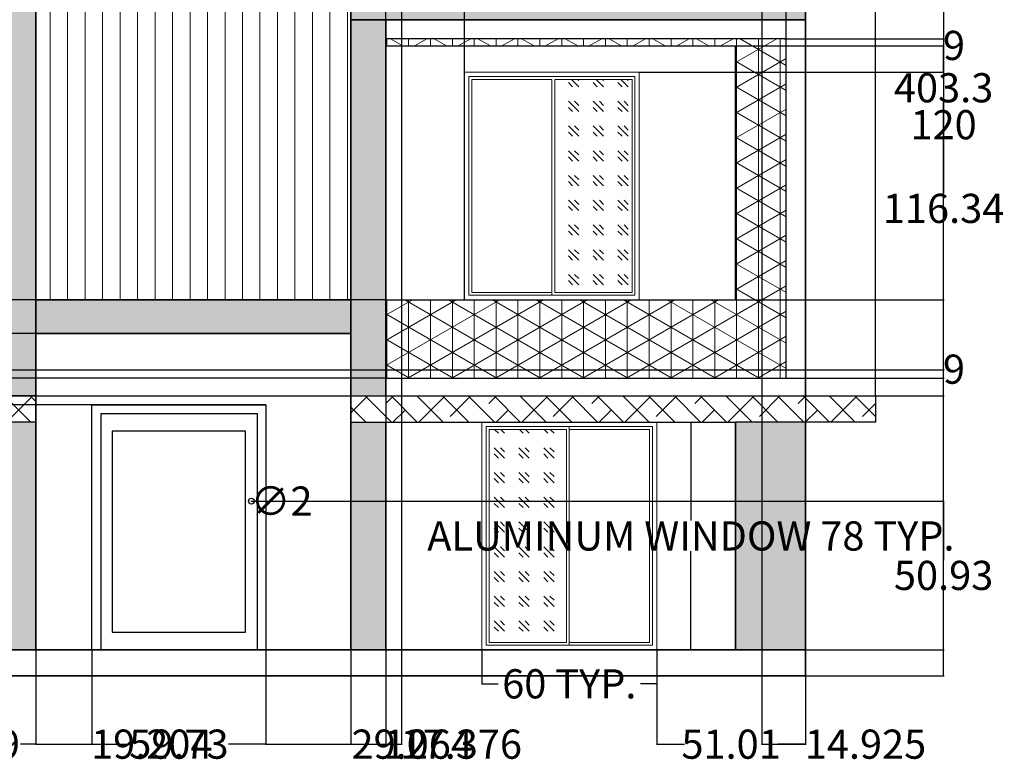
# Model space of a CAD drawing. Units: inches. Extents: x -37 to 519, y -28 to 435.
# Tile 2 of 3: x 182 to 519, y -28 to 227. Entities that reach past the tile are written whole.
import ezdxf

# ---------------------------------------------------------------- set-up
doc = ezdxf.new("R2010")
doc.units = ezdxf.units.IN
doc.header["$MEASUREMENT"] = 0
for name, color, linetype, lineweight in [('A-ANNO-DIMS', 2, 'Continuous', 18), ('A-DOOR', 3, 'Continuous', 25), ('A-GLAZ', 4, 'Continuous', 18), ('A-GLAZ-PATT', 9, 'Continuous', 13), ('A-WALL', 7, 'Continuous', 35), ('A-WALL-PATT', 8, 'Continuous', 13), ('A-WALL-TRIM', 7, 'Continuous', 25), ('A-WALL-TRIM-PATT', 8, 'Continuous', 13)]:
    doc.layers.add(name, color=color, linetype=linetype, lineweight=lineweight)
doc.styles.get("Standard").update_dxf_attribs({"font": 'arial.ttf'})
doc.dimstyles.get("Standard").update_dxf_attribs({"dimtxt": 10, "dimasz": 0.18, "dimexe": 0.18, "dimexo": 0.0625, "dimgap": 0.09, "dimtad": 0, "dimtih": 1, "dimtoh": 1, "dimdec": 0, "dimzin": 0, "dimdsep": 46, "dimlunit": 3, "dimtxsty": 'Standard', "dimcen": 0.09, "dimadec": 0, "dimazin": 0, "dimtfac": 1, "dimtdec": 0, "dimtofl": 0, "dimtmove": 0, "dimatfit": 3, "dimfxl": 1, "dimtolj": 1, "dimtzin": 0, "dimarcsym": 0})

# ---------------------------------------------------------------- blocks, each defined once
blk = doc.blocks.new('WIN-ALUM-60X78-ELEV')
for p, q in [((1.5, 1.5), (1.5, 76.5)), ((1.5, 76.5), (30, 76.5)), ((30, 1.5), (30, 76.5)), ((30, 76.5), (58.5, 76.5)), ((58.5, 76.5), (58.5, 1.5)), ((30, 1.5), (1.5, 1.5)), ((58.5, 1.5), (30, 1.5))]:
    blk.add_line(p, q)
blk.add_lwpolyline([(0, 0), (0, 78), (60, 78), (60, 0)], close=True)
for points in [[(29, 75.5), (29, 2.5), (2.5, 2.5), (2.5, 75.5), (29, 75.5)], [(30, 75.5), (57.5, 75.5), (57.5, 2.5), (30, 2.5)]]:
    blk.add_lwpolyline(points)
blk = doc.blocks.new('*D5')
at = {"layer": 'A-ANNO-DIMS', "color": 0, "lineweight": -2, "transparency": 16777216}
for p, q in [((400.18, 88.65), (412, 88.65)), ((411.82, 88.47), (411.82, 54.92)), ((411.82, 10.83), (411.82, 44.39)), ((400.18, 10.65), (412, 10.65))]:
    blk.add_line(p, q, dxfattribs=at)
at = {"layer": 'A-ANNO-DIMS', "color": 0, "transparency": 16777216}
for points in [[(411.79, 88.47), (411.85, 88.47), (411.82, 88.65)], [(411.79, 10.83), (411.85, 10.83), (411.82, 10.65)]]:
    blk.add_solid(points, dxfattribs=at)
at = {"layer": 'Defpoints', "color": 0, "transparency": 16777216}
for p in [(400.12, 88.65), (411.82, 88.65), (400.12, 10.65)]:
    blk.add_point(p, dxfattribs=at)
at = {"layer": 'A-ANNO-DIMS', "color": 0, "transparency": 16777216, "insert": (411.82, 49.65), "char_height": 10, "attachment_point": 5}
blk.add_mtext('\\A1;ALUMINUM WINDOW 78 TYP.', dxfattribs=at)
blk = doc.blocks.new('*D6')
at = {"layer": 'A-ANNO-DIMS', "color": 0, "lineweight": -2, "transparency": 16777216}
for p, q in [((340.12, 10.59), (340.12, -1.23)), ((400.12, 10.59), (400.12, -1.23)), ((340.3, -1.05), (345.66, -1.05)), ((399.94, -1.05), (394.58, -1.05))]:
    blk.add_line(p, q, dxfattribs=at)
at = {"layer": 'A-ANNO-DIMS', "color": 0, "transparency": 16777216}
for points in [[(340.3, -1.02), (340.3, -1.08), (340.12, -1.05)], [(399.94, -1.02), (399.94, -1.08), (400.12, -1.05)]]:
    blk.add_solid(points, dxfattribs=at)
at = {"layer": 'Defpoints', "color": 0, "transparency": 16777216}
for p in [(340.12, 10.65), (400.12, 10.65), (400.12, -1.05)]:
    blk.add_point(p, dxfattribs=at)
at = {"layer": 'A-ANNO-DIMS', "color": 0, "transparency": 16777216, "insert": (370.12, -1.05), "char_height": 10, "attachment_point": 5}
blk.add_mtext('\\A1;60 TYP.', dxfattribs=at)
blk = doc.blocks.new('*D7')
at = {"layer": 'A-ANNO-DIMS', "color": 0, "lineweight": -2, "transparency": 16777216}
for p, q in [((7.62, 97.72), (7.62, 428.56)), ((7.8, 428.38), (224.17, 428.38)), ((474.95, 428.38), (258.57, 428.38)), ((475.13, 97.72), (475.13, 428.56))]:
    blk.add_line(p, q, dxfattribs=at)
at = {"layer": 'A-ANNO-DIMS', "color": 0, "transparency": 16777216}
for points in [[(7.8, 428.41), (7.8, 428.35), (7.62, 428.38)], [(474.95, 428.41), (474.95, 428.35), (475.13, 428.38)]]:
    blk.add_solid(points, dxfattribs=at)
at = {"layer": 'Defpoints', "color": 0, "transparency": 16777216}
for p in [(475.13, 428.38), (7.62, 97.65), (475.13, 97.65)]:
    blk.add_point(p, dxfattribs=at)
at = {"layer": 'A-ANNO-DIMS', "color": 0, "transparency": 16777216, "insert": (241.37, 428.38), "char_height": 10, "attachment_point": 5}
blk.add_mtext('\\A1;467.5', dxfattribs=at)
blk = doc.blocks.new('*D8')
at = {"layer": 'A-ANNO-DIMS', "color": 0, "lineweight": -2, "transparency": 16777216}
for p, q in [((451.19, 404.99), (498.7, 404.99)), ((498.52, 404.81), (498.52, 208.52)), ((498.52, 1.83), (498.52, 198.12)), ((451.19, 1.65), (498.7, 1.65))]:
    blk.add_line(p, q, dxfattribs=at)
at = {"layer": 'A-ANNO-DIMS', "color": 0, "transparency": 16777216}
for points in [[(498.49, 404.81), (498.55, 404.81), (498.52, 404.99)], [(498.49, 1.83), (498.55, 1.83), (498.52, 1.65)]]:
    blk.add_solid(points, dxfattribs=at)
at = {"layer": 'Defpoints', "color": 0, "transparency": 16777216}
for p in [(451.13, 404.99), (498.52, 404.99), (451.13, 1.65)]:
    blk.add_point(p, dxfattribs=at)
at = {"layer": 'A-ANNO-DIMS', "color": 0, "transparency": 16777216, "insert": (498.52, 203.32), "char_height": 10, "attachment_point": 5}
blk.add_mtext('\\A1;403.3', dxfattribs=at)
blk = doc.blocks.new('*D11')
at = {"layer": 'A-ANNO-DIMS', "color": 0, "lineweight": -2, "transparency": 16777216}
for p, q in [((142.13, 10.59), (142.13, -21.92)), ((187.13, 10.59), (187.13, -21.92)), ((142.31, -21.74), (147.46, -21.74)), ((186.95, -21.74), (181.8, -21.74))]:
    blk.add_line(p, q, dxfattribs=at)
at = {"layer": 'A-ANNO-DIMS', "color": 0, "transparency": 16777216}
for points in [[(142.31, -21.71), (142.31, -21.77), (142.13, -21.74)], [(186.95, -21.71), (186.95, -21.77), (187.13, -21.74)]]:
    blk.add_solid(points, dxfattribs=at)
at = {"layer": 'Defpoints', "color": 0, "transparency": 16777216}
for p in [(142.13, 10.65), (187.13, 10.65), (187.13, -21.74)]:
    blk.add_point(p, dxfattribs=at)
at = {"layer": 'A-ANNO-DIMS', "color": 0, "transparency": 16777216, "insert": (164.63, -21.74), "char_height": 10, "attachment_point": 5}
blk.add_mtext('\\A1;44.99', dxfattribs=at)
blk = doc.blocks.new('*D12')
at = {"layer": 'A-ANNO-DIMS', "color": 0, "lineweight": -2, "transparency": 16777216}
for p, q in [((187.13, 10.59), (187.13, -21.92)), ((206.33, 10.59), (206.33, -21.92)), ((187.31, -21.74), (206.15, -21.74)), ((206.33, -21.74), (206.51, -21.74))]:
    blk.add_line(p, q, dxfattribs=at)
at = {"layer": 'A-ANNO-DIMS', "color": 0, "transparency": 16777216}
for points in [[(187.31, -21.71), (187.31, -21.77), (187.13, -21.74)], [(206.15, -21.71), (206.15, -21.77), (206.33, -21.74)]]:
    blk.add_solid(points, dxfattribs=at)
at = {"layer": 'Defpoints', "color": 0, "transparency": 16777216}
for p in [(187.13, 10.65), (206.33, 10.65), (206.33, -21.74)]:
    blk.add_point(p, dxfattribs=at)
at = {"layer": 'A-ANNO-DIMS', "color": 0, "transparency": 16777216, "insert": (226.87, -21.74), "char_height": 10, "attachment_point": 5}
blk.add_mtext('\\A1;19.204', dxfattribs=at)
blk = doc.blocks.new('*D13')
at = {"layer": 'A-ANNO-DIMS', "color": 0, "lineweight": -2, "transparency": 16777216}
for p, q in [((206.33, 10.59), (206.33, -21.92)), ((266.06, 10.59), (266.06, -21.92)), ((206.51, -21.74), (219.23, -21.74)), ((265.88, -21.74), (253.16, -21.74))]:
    blk.add_line(p, q, dxfattribs=at)
at = {"layer": 'A-ANNO-DIMS', "color": 0, "transparency": 16777216}
for points in [[(206.51, -21.71), (206.51, -21.77), (206.33, -21.74)], [(265.88, -21.71), (265.88, -21.77), (266.06, -21.74)]]:
    blk.add_solid(points, dxfattribs=at)
at = {"layer": 'Defpoints', "color": 0, "transparency": 16777216}
for p in [(206.33, 10.65), (266.06, 10.65), (266.06, -21.74)]:
    blk.add_point(p, dxfattribs=at)
at = {"layer": 'A-ANNO-DIMS', "color": 0, "transparency": 16777216, "insert": (236.2, -21.74), "char_height": 10, "attachment_point": 5}
blk.add_mtext('\\A1;59.73', dxfattribs=at)
blk = doc.blocks.new('*D14')
at = {"layer": 'A-ANNO-DIMS', "color": 0, "lineweight": -2, "transparency": 16777216}
for p, q in [((266.06, 10.59), (266.06, -21.92)), ((295.13, 10.59), (295.13, -21.92)), ((266.24, -21.74), (294.95, -21.74)), ((295.13, -21.74), (295.31, -21.74))]:
    blk.add_line(p, q, dxfattribs=at)
at = {"layer": 'A-ANNO-DIMS', "color": 0, "transparency": 16777216}
for points in [[(266.24, -21.71), (266.24, -21.77), (266.06, -21.74)], [(294.95, -21.71), (294.95, -21.77), (295.13, -21.74)]]:
    blk.add_solid(points, dxfattribs=at)
at = {"layer": 'Defpoints', "color": 0, "transparency": 16777216}
for p in [(266.06, 10.65), (295.13, 10.65), (295.13, -21.74)]:
    blk.add_point(p, dxfattribs=at)
at = {"layer": 'A-ANNO-DIMS', "color": 0, "transparency": 16777216, "insert": (316.22, -21.74), "char_height": 10, "attachment_point": 5}
blk.add_mtext('\\A1;29.064', dxfattribs=at)
blk = doc.blocks.new('*D15')
at = {"layer": 'A-ANNO-DIMS', "color": 0, "lineweight": -2, "transparency": 16777216}
for p, q in [((400.12, 10.59), (400.12, -21.92)), ((451.13, 10.59), (451.13, -21.92)), ((400.3, -21.74), (409.63, -21.74)), ((450.95, -21.74), (441.62, -21.74))]:
    blk.add_line(p, q, dxfattribs=at)
at = {"layer": 'A-ANNO-DIMS', "color": 0, "transparency": 16777216}
for points in [[(400.3, -21.71), (400.3, -21.77), (400.12, -21.74)], [(450.95, -21.71), (450.95, -21.77), (451.13, -21.74)]]:
    blk.add_solid(points, dxfattribs=at)
at = {"layer": 'Defpoints', "color": 0, "transparency": 16777216}
for p in [(400.12, 10.65), (451.13, 10.65), (451.13, -21.74)]:
    blk.add_point(p, dxfattribs=at)
at = {"layer": 'A-ANNO-DIMS', "color": 0, "transparency": 16777216, "insert": (425.62, -21.74), "char_height": 10, "attachment_point": 5}
blk.add_mtext('\\A1;51.01', dxfattribs=at)
blk = doc.blocks.new('*D16')
at = {"layer": 'A-ANNO-DIMS', "color": 0, "lineweight": -2, "transparency": 16777216}
for p, q in [((206.27, 94.65), (-15.95, 94.65)), ((-15.77, 94.47), (-15.77, 57.85)), ((-15.77, 10.83), (-15.77, 47.46)), ((206.27, 10.65), (-15.95, 10.65))]:
    blk.add_line(p, q, dxfattribs=at)
at = {"layer": 'A-ANNO-DIMS', "color": 0, "transparency": 16777216}
for points in [[(-15.8, 94.47), (-15.74, 94.47), (-15.77, 94.65)], [(-15.8, 10.83), (-15.74, 10.83), (-15.77, 10.65)]]:
    blk.add_solid(points, dxfattribs=at)
at = {"layer": 'Defpoints', "color": 0, "transparency": 16777216}
for p in [(-15.77, 94.65), (206.33, 94.65), (206.33, 10.65)]:
    blk.add_point(p, dxfattribs=at)
at = {"layer": 'A-ANNO-DIMS', "color": 0, "transparency": 16777216, "insert": (-15.77, 52.65), "char_height": 10, "attachment_point": 5}
blk.add_mtext('\\A1;84', dxfattribs=at)
blk = doc.blocks.new('*D17')
at = {"layer": 'A-ANNO-DIMS', "color": 0, "lineweight": -2, "transparency": 16777216}
for p, q in [((261.13, 61.58), (498.7, 61.58)), ((498.52, 61.4), (498.52, 41.32)), ((498.52, 10.83), (498.52, 30.92)), ((266.13, 10.65), (498.7, 10.65))]:
    blk.add_line(p, q, dxfattribs=at)
at = {"layer": 'A-ANNO-DIMS', "color": 0, "transparency": 16777216}
for points in [[(498.49, 61.4), (498.55, 61.4), (498.52, 61.58)], [(498.49, 10.83), (498.55, 10.83), (498.52, 10.65)]]:
    blk.add_solid(points, dxfattribs=at)
at = {"layer": 'Defpoints', "color": 0, "transparency": 16777216}
for p in [(261.06, 61.58), (266.06, 10.65), (498.52, 10.65)]:
    blk.add_point(p, dxfattribs=at)
at = {"layer": 'A-ANNO-DIMS', "color": 0, "transparency": 16777216, "insert": (498.52, 36.12), "char_height": 10, "attachment_point": 5}
blk.add_mtext('\\A1;50.93', dxfattribs=at)
blk = doc.blocks.new('*D27')
at = {"layer": 'A-ANNO-DIMS', "color": 0, "lineweight": -2, "transparency": 16777216}
for p, q in [((295.06, 119.05), (-15.95, 119.05)), ((-15.77, 118.87), (-15.77, 112.05)), ((-15.77, 94.83), (-15.77, 101.65)), ((266, 94.65), (-15.95, 94.65))]:
    blk.add_line(p, q, dxfattribs=at)
at = {"layer": 'A-ANNO-DIMS', "color": 0, "transparency": 16777216}
for points in [[(-15.8, 118.87), (-15.74, 118.87), (-15.77, 119.05)], [(-15.8, 94.83), (-15.74, 94.83), (-15.77, 94.65)]]:
    blk.add_solid(points, dxfattribs=at)
at = {"layer": 'Defpoints', "color": 0, "transparency": 16777216}
for p in [(-15.77, 119.05), (295.13, 119.05), (266.06, 94.65)]:
    blk.add_point(p, dxfattribs=at)
at = {"layer": 'A-ANNO-DIMS', "color": 0, "transparency": 16777216, "insert": (-15.77, 106.85), "char_height": 10, "attachment_point": 5}
blk.add_mtext('\\A1;24.393', dxfattribs=at)
blk = doc.blocks.new('*D31')
at = {"layer": 'A-ANNO-DIMS', "color": 0, "lineweight": -2, "transparency": 16777216}
for p, q in [((175.19, 106.65), (498.7, 106.65)), ((498.52, 106.65), (498.52, 106.83)), ((498.52, 106.83), (498.7, 106.83)), ((498.52, 97.83), (498.52, 106.47)), ((175.19, 97.65), (498.7, 97.65))]:
    blk.add_line(p, q, dxfattribs=at)
at = {"layer": 'A-ANNO-DIMS', "color": 0, "transparency": 16777216}
for points in [[(498.49, 106.47), (498.55, 106.47), (498.52, 106.65)], [(498.49, 97.83), (498.55, 97.83), (498.52, 97.65)]]:
    blk.add_solid(points, dxfattribs=at)
at = {"layer": 'Defpoints', "color": 0, "transparency": 16777216}
for p in [(175.13, 106.65), (498.52, 106.65), (175.13, 97.65)]:
    blk.add_point(p, dxfattribs=at)
at = {"layer": 'A-ANNO-DIMS', "color": 0, "transparency": 16777216, "insert": (502.08, 106.83), "char_height": 10, "attachment_point": 5}
blk.add_mtext('\\A1;9', dxfattribs=at)
blk = doc.blocks.new('*D32')
at = {"layer": 'A-ANNO-DIMS', "color": 0, "lineweight": -2, "transparency": 16777216}
for p, q in [((394.2, 250.65), (498.7, 250.65)), ((498.52, 250.47), (498.52, 195.85)), ((498.52, 130.83), (498.52, 185.46)), ((394.2, 130.65), (498.7, 130.65))]:
    blk.add_line(p, q, dxfattribs=at)
at = {"layer": 'A-ANNO-DIMS', "color": 0, "transparency": 16777216}
for points in [[(498.49, 250.47), (498.55, 250.47), (498.52, 250.65)], [(498.49, 130.83), (498.55, 130.83), (498.52, 130.65)]]:
    blk.add_solid(points, dxfattribs=at)
at = {"layer": 'Defpoints', "color": 0, "transparency": 16777216}
for p in [(394.13, 250.65), (498.52, 250.65), (394.13, 130.65)]:
    blk.add_point(p, dxfattribs=at)
at = {"layer": 'A-ANNO-DIMS', "color": 0, "transparency": 16777216, "insert": (498.52, 190.65), "char_height": 10, "attachment_point": 5}
blk.add_mtext('\\A1;120', dxfattribs=at)
blk = doc.blocks.new('*D40')
at = {"layer": 'A-ANNO-DIMS', "color": 0, "lineweight": -2, "transparency": 16777216}
for p, q in [((295.13, 393.45), (295.13, -21.92)), ((312.5, 393.45), (312.5, -21.92)), ((295.31, -21.74), (312.32, -21.74)), ((312.5, -21.74), (312.68, -21.74))]:
    blk.add_line(p, q, dxfattribs=at)
at = {"layer": 'A-ANNO-DIMS', "color": 0, "transparency": 16777216}
for points in [[(295.31, -21.71), (295.31, -21.77), (295.13, -21.74)], [(312.32, -21.71), (312.32, -21.77), (312.5, -21.74)]]:
    blk.add_solid(points, dxfattribs=at)
at = {"layer": 'Defpoints', "color": 0, "transparency": 16777216}
for p in [(295.13, 393.51), (312.5, 393.51), (312.5, -21.74)]:
    blk.add_point(p, dxfattribs=at)
at = {"layer": 'A-ANNO-DIMS', "color": 0, "transparency": 16777216, "insert": (333.06, -21.74), "char_height": 10, "attachment_point": 5}
blk.add_mtext('\\A1;17.376', dxfattribs=at)
blk = doc.blocks.new('*D41')
at = {"layer": 'A-ANNO-DIMS', "color": 0, "lineweight": -2, "transparency": 16777216}
for p, q in [((436.2, 393.45), (436.2, -21.92)), ((451.13, 393.45), (451.13, -21.92)), ((436.38, -21.74), (450.95, -21.74)), ((451.13, -21.74), (451.31, -21.74))]:
    blk.add_line(p, q, dxfattribs=at)
at = {"layer": 'A-ANNO-DIMS', "color": 0, "transparency": 16777216}
for points in [[(436.38, -21.71), (436.38, -21.77), (436.2, -21.74)], [(450.95, -21.71), (450.95, -21.77), (451.13, -21.74)]]:
    blk.add_solid(points, dxfattribs=at)
at = {"layer": 'Defpoints', "color": 0, "transparency": 16777216}
for p in [(436.2, 393.51), (451.13, 393.51), (451.13, -21.74)]:
    blk.add_point(p, dxfattribs=at)
at = {"layer": 'A-ANNO-DIMS', "color": 0, "transparency": 16777216, "insert": (471.72, -21.74), "char_height": 10, "attachment_point": 5}
blk.add_mtext('\\A1;14.925', dxfattribs=at)
blk = doc.blocks.new('*D44')
at = {"layer": 'A-ANNO-DIMS', "color": 0, "lineweight": -2, "transparency": 16777216}
for p, q in [((307.13, 220.19), (307.13, 428.56)), ((307.31, 428.38), (359.36, 428.38)), ((444.36, 428.38), (392.3, 428.38)), ((444.54, 220.19), (444.54, 428.56))]:
    blk.add_line(p, q, dxfattribs=at)
at = {"layer": 'A-ANNO-DIMS', "color": 0, "transparency": 16777216}
for points in [[(307.31, 428.41), (307.31, 428.35), (307.13, 428.38)], [(444.36, 428.41), (444.36, 428.35), (444.54, 428.38)]]:
    blk.add_solid(points, dxfattribs=at)
at = {"layer": 'Defpoints', "color": 0, "transparency": 16777216}
for p in [(444.54, 428.38), (307.13, 220.13), (444.54, 220.13)]:
    blk.add_point(p, dxfattribs=at)
at = {"layer": 'A-ANNO-DIMS', "color": 0, "transparency": 16777216, "insert": (375.83, 428.38), "char_height": 10, "attachment_point": 5}
blk.add_mtext('\\A1;137.4', dxfattribs=at)
blk = doc.blocks.new('*D45')
at = {"layer": 'A-ANNO-DIMS', "color": 0, "lineweight": -2, "transparency": 16777216}
for p, q in [((444.6, 220.13), (498.7, 220.13)), ((498.52, 219.95), (498.52, 167.16)), ((498.52, 103.97), (498.52, 156.76)), ((444.6, 103.79), (498.7, 103.79))]:
    blk.add_line(p, q, dxfattribs=at)
at = {"layer": 'A-ANNO-DIMS', "color": 0, "transparency": 16777216}
for points in [[(498.49, 219.95), (498.55, 219.95), (498.52, 220.13)], [(498.49, 103.97), (498.55, 103.97), (498.52, 103.79)]]:
    blk.add_solid(points, dxfattribs=at)
at = {"layer": 'Defpoints', "color": 0, "transparency": 16777216}
for p in [(444.54, 220.13), (498.52, 220.13), (444.54, 103.79)]:
    blk.add_point(p, dxfattribs=at)
at = {"layer": 'A-ANNO-DIMS', "color": 0, "transparency": 16777216, "insert": (498.52, 161.96), "char_height": 10, "attachment_point": 5}
blk.add_mtext('\\A1;116.34', dxfattribs=at)
blk = doc.blocks.new('*D46')
at = {"layer": 'A-ANNO-DIMS', "color": 0, "lineweight": -2, "transparency": 16777216}
for p, q in [((307.06, 130.65), (-15.95, 130.65)), ((-15.77, 130.47), (-15.77, 122.42)), ((-15.77, 103.97), (-15.77, 112.03)), ((307.06, 103.79), (-15.95, 103.79))]:
    blk.add_line(p, q, dxfattribs=at)
at = {"layer": 'A-ANNO-DIMS', "color": 0, "transparency": 16777216}
for points in [[(-15.8, 130.47), (-15.74, 130.47), (-15.77, 130.65)], [(-15.8, 103.97), (-15.74, 103.97), (-15.77, 103.79)]]:
    blk.add_solid(points, dxfattribs=at)
at = {"layer": 'Defpoints', "color": 0, "transparency": 16777216}
for p in [(307.13, 130.65), (-15.77, 103.79), (307.13, 103.79)]:
    blk.add_point(p, dxfattribs=at)
at = {"layer": 'A-ANNO-DIMS', "color": 0, "transparency": 16777216, "insert": (-15.77, 117.22), "char_height": 10, "attachment_point": 5}
blk.add_mtext('\\A1;26.86', dxfattribs=at)
blk = doc.blocks.new('*D47')
at = {"layer": 'A-ANNO-DIMS', "color": 0, "lineweight": -2, "transparency": 16777216}
for p, q in [((307.13, 130.72), (307.13, 428.56)), ((307.31, 428.38), (333.95, 428.38)), ((334.13, 130.72), (334.13, 428.56)), ((334.13, 428.38), (334.31, 428.38))]:
    blk.add_line(p, q, dxfattribs=at)
at = {"layer": 'A-ANNO-DIMS', "color": 0, "transparency": 16777216}
for points in [[(307.31, 428.41), (307.31, 428.35), (307.13, 428.38)], [(333.95, 428.41), (333.95, 428.35), (334.13, 428.38)]]:
    blk.add_solid(points, dxfattribs=at)
at = {"layer": 'Defpoints', "color": 0, "transparency": 16777216}
for p in [(334.13, 428.38), (307.13, 130.65), (334.13, 130.65)]:
    blk.add_point(p, dxfattribs=at)
at = {"layer": 'A-ANNO-DIMS', "color": 0, "transparency": 16777216, "insert": (355.25, 428.38), "char_height": 10, "attachment_point": 5}
blk.add_mtext('\\A1;27.007', dxfattribs=at)
blk = doc.blocks.new('*D48')
at = {"layer": 'A-ANNO-DIMS', "color": 0, "lineweight": -2, "transparency": 16777216}
for p, q in [((295.13, 226.59), (295.13, -21.92)), ((307.13, 226.59), (307.13, -21.92)), ((295.31, -21.74), (306.95, -21.74)), ((307.13, -21.74), (307.31, -21.74))]:
    blk.add_line(p, q, dxfattribs=at)
at = {"layer": 'A-ANNO-DIMS', "color": 0, "transparency": 16777216}
for points in [[(295.31, -21.71), (295.31, -21.77), (295.13, -21.74)], [(306.95, -21.71), (306.95, -21.77), (307.13, -21.74)]]:
    blk.add_solid(points, dxfattribs=at)
at = {"layer": 'Defpoints', "color": 0, "transparency": 16777216}
for p in [(295.13, 226.65), (307.13, 226.65), (307.13, -21.74)]:
    blk.add_point(p, dxfattribs=at)
at = {"layer": 'A-ANNO-DIMS', "color": 0, "transparency": 16777216, "insert": (314.04, -21.74), "char_height": 10, "attachment_point": 5}
blk.add_mtext('\\A1;12', dxfattribs=at)
blk = doc.blocks.new('*D49')
at = {"layer": 'A-ANNO-DIMS', "color": 0, "lineweight": -2, "transparency": 16777216}
for p, q in [((427.19, 217.65), (498.7, 217.65)), ((498.52, 217.65), (498.52, 217.83)), ((498.52, 217.83), (498.7, 217.83)), ((498.52, 208.83), (498.52, 217.47)), ((394.2, 208.65), (498.7, 208.65))]:
    blk.add_line(p, q, dxfattribs=at)
at = {"layer": 'A-ANNO-DIMS', "color": 0, "transparency": 16777216}
for points in [[(498.49, 217.47), (498.55, 217.47), (498.52, 217.65)], [(498.49, 208.83), (498.55, 208.83), (498.52, 208.65)]]:
    blk.add_solid(points, dxfattribs=at)
at = {"layer": 'Defpoints', "color": 0, "transparency": 16777216}
for p in [(427.13, 217.65), (498.52, 217.65), (394.13, 208.65)]:
    blk.add_point(p, dxfattribs=at)
at = {"layer": 'A-ANNO-DIMS', "color": 0, "transparency": 16777216, "insert": (502.08, 217.83), "char_height": 10, "attachment_point": 5}
blk.add_mtext('\\A1;9', dxfattribs=at)
blk = doc.blocks.new('*D50')
at = {"layer": 'A-ANNO-DIMS', "color": 0, "lineweight": -2, "transparency": 16777216}
for p, q in [((260.97, 61.58), (261.15, 61.58)), ((261.06, 61.49), (261.06, 61.67)), ((262.66, 61.61), (262.24, 61.6))]:
    blk.add_line(p, q, dxfattribs=at)
at = {"layer": 'A-ANNO-DIMS', "color": 0, "transparency": 16777216}
blk.add_solid([(262.24, 61.63), (262.24, 61.57), (262.06, 61.6)], dxfattribs=at)
at = {"layer": 'Defpoints', "color": 0, "transparency": 16777216}
for p in [(260.06, 61.56), (262.06, 61.6)]:
    blk.add_point(p, dxfattribs=at)
at = {"layer": 'A-ANNO-DIMS', "color": 0, "transparency": 16777216, "insert": (271.42, 61.61), "char_height": 10, "attachment_point": 5}
blk.add_mtext('\\A1;∅2', dxfattribs=at)

msp = doc.modelspace()

# ---------------------------------------------------------------- hatches: boundary and pattern name
at = {"layer": 'A-GLAZ-PATT'}
h = msp.add_hatch(dxfattribs=at)
h.set_pattern_fill('GOST_GLASS', color=256, angle=90)
h.set_pattern_definition([(135, (0, 0), (5e-16, 8.48528), [5, -7]), (135, (1e-16, 2.1213), (5e-16, 8.48528), [2, -10]), (135, (-2.1213, 1e-16), (5e-16, 8.48528), [2, -10])])
h.paths.add_polyline_path([(112.1341, 206.153), (84.6341, 206.153), (84.6341, 133.153), (112.1341, 133.153)])
h.paths.add_polyline_path([(139.6341, 86.153), (113.1341, 86.153), (113.1341, 13.153), (139.6341, 13.153)])
h.paths.add_polyline_path([(369.1204, 86.153), (342.6204, 86.153), (342.6204, 13.153), (369.1204, 13.153)])
h.paths.add_polyline_path([(391.6341, 206.153), (365.1341, 206.153), (365.1341, 133.153), (391.6341, 133.153)])
h.paths.add_polyline_path([(78.851, 283.8209), (34.1272, 283.8209), (34.1272, 259.7765), (78.851, 259.7765)])
at = {"layer": 'A-WALL-PATT'}
h = msp.add_hatch(color=256, dxfattribs=at)
h.dxf.hatch_style = 1
h.paths.add_polyline_path([(451.1272, 370.653), (295.1272, 370.653), (295.1272, 226.653), (451.1272, 226.653)])
h.paths.add_polyline_path([(319.1272, 346.653), (427.1272, 346.653), (427.1272, 250.653), (319.1272, 250.653)], flags=16)
h.paths.add_polyline_path([(334.1341, 346.653), (394.1341, 346.653), (394.1341, 250.653), (334.1341, 250.653)], flags=0)
h.paths.add_polyline_path([(335.6341, 345.153), (364.1341, 345.153), (392.6341, 345.153), (392.6341, 252.153), (364.1341, 252.153), (335.6341, 252.153)], flags=0)
h.paths.add_polyline_path([(336.6341, 344.153), (364.1341, 344.153), (364.1341, 253.153), (336.6341, 253.153)], flags=0)
h.paths.add_polyline_path([(365.1341, 344.153), (391.6341, 344.153), (391.6341, 253.153), (365.1341, 253.153)], flags=0)
h.paths.add_polyline_path([(187.1272, 370.653), (175.1272, 370.653), (175.1272, 256.7765), (31.1272, 256.7765), (31.1272, 97.653), (55.1272, 97.653), (55.1272, 106.653), (175.1272, 106.653), (175.1272, 97.653), (187.1272, 97.653)])
h.paths.add_polyline_path([(175.1272, 208.7765), (175.1272, 130.653), (55.1272, 130.653), (55.1272, 208.7765)], flags=16)
h.paths.add_polyline_path([(142.1341, 208.653), (142.1341, 130.653), (82.1341, 130.653), (82.1341, 208.653)], flags=0)
h.paths.add_polyline_path([(112.1341, 207.153), (140.6341, 207.153), (140.6341, 132.153), (112.1341, 132.153), (83.6341, 132.153), (83.6341, 207.153)], flags=0)
h.paths.add_polyline_path([(112.1341, 133.153), (84.6341, 133.153), (84.6341, 206.153), (112.1341, 206.153)], flags=0)
h.paths.add_polyline_path([(139.6341, 206.153), (139.6341, 133.153), (113.1341, 133.153), (113.1341, 206.153)], flags=0)
h.paths.add_polyline_path([(187.1272, 88.653), (175.1272, 88.653), (175.1272, 10.653), (187.1272, 10.653)])
h.paths.add_polyline_path([(307.1272, 88.653), (295.1272, 88.653), (295.1272, 10.653), (307.1272, 10.653)])
h.paths.add_polyline_path([(451.1272, 88.653), (427.1272, 88.653), (427.1272, 10.653), (451.1272, 10.653)])
h = msp.add_hatch(dxfattribs=at)
h.set_pattern_fill('_USER', color=256, scale=6, angle=90, pattern_type=0)
h.set_pattern_definition([(90, (0, 0), (-6, 4e-16), [])])
h.paths.add_polyline_path([(295.1272, 353.3062), (187.1272, 353.3062), (187.1272, 130.653), (295.1272, 130.653)])
h = msp.add_hatch(color=256, dxfattribs=at)
h.dxf.hatch_style = 1
h.paths.add_polyline_path([(307.1272, 226.653), (295.1272, 226.653), (295.1272, 97.653), (307.1272, 97.653), (307.1272, 130.653)])
h.paths.add_polyline_path([(55.1272, 88.653), (31.1272, 88.653), (31.1272, 10.653), (55.1272, 10.653)])
at = {"layer": 'A-WALL-TRIM-PATT'}
h = msp.add_hatch(dxfattribs=at)
h.set_pattern_fill('NET3', color=256, scale=60, angle=90)
h.paths.add_polyline_path([(444.5372, 220.1322), (307.1272, 220.1322), (307.1272, 217.653), (427.1272, 217.653), (427.1272, 130.653), (307.1272, 130.653), (307.1272, 103.7936), (444.5372, 103.7936)])
h = msp.add_hatch(color=256, dxfattribs=at)
h.dxf.hatch_style = 1
h.paths.add_polyline_path([(295.1272, 130.653), (187.1272, 130.653), (187.1272, 119.0462), (295.1272, 119.0462)])
h = msp.add_hatch(dxfattribs=at)
h.set_pattern_fill('ANSI38', color=256, scale=50, angle=90)
h.paths.add_polyline_path([(187.1272, 97.653), (55.1272, 97.653), (7.6202, 97.653), (7.6202, 88.653), (55.1272, 88.653), (187.1272, 88.653)])
h.paths.add_polyline_path([(475.1272, 97.653), (427.1272, 97.653), (295.1272, 97.653), (295.1272, 88.653), (427.1272, 88.653), (475.1272, 88.653)])

# ---------------------------------------------------------------- linework, layer by layer
at = {"layer": 'A-DOOR'}
msp.add_lwpolyline([(209.3316, 10.653), (206.3316, 10.653), (206.3316, 94.653), (266.063, 94.653), (266.063, 10.653), (263.063, 10.653)], dxfattribs=at)
for points in [[(263.063, 91.63), (263.063, 10.653), (209.5485, 10.653), (209.5485, 91.63)], [(259.063, 16.653), (259.063, 85.63), (213.3316, 85.63), (213.3316, 16.653)]]:
    msp.add_lwpolyline(points, close=True, dxfattribs=at)
msp.add_circle((261.063, 61.5817), 1, dxfattribs=at)
at = {"layer": 'A-GLAZ'}
for p, q in [((364.1341, 207.153), (335.6341, 207.153)), ((335.6341, 207.153), (335.6341, 132.153)), ((364.1341, 207.153), (335.6341, 207.153)), ((335.6341, 207.153), (335.6341, 132.153)), ((364.1341, 207.153), (335.6341, 207.153)), ((335.6341, 207.153), (335.6341, 132.153)), ((364.1341, 207.153), (335.6341, 207.153)), ((335.6341, 207.153), (335.6341, 132.153)), ((392.6341, 207.153), (364.1341, 207.153)), ((392.6341, 207.153), (364.1341, 207.153)), ((392.6341, 207.153), (364.1341, 207.153)), ((392.6341, 207.153), (364.1341, 207.153)), ((364.1341, 132.153), (364.1341, 206.153)), ((364.1341, 132.153), (364.1341, 206.153)), ((364.1341, 132.153), (364.1341, 206.153)), ((364.1341, 132.153), (364.1341, 206.153)), ((392.6341, 132.153), (392.6341, 207.153)), ((392.6341, 132.153), (392.6341, 207.153)), ((392.6341, 132.153), (392.6341, 207.153)), ((392.6341, 132.153), (392.6341, 207.153)), ((335.6341, 132.153), (364.1341, 132.153)), ((335.6341, 132.153), (364.1341, 132.153)), ((335.6341, 132.153), (364.1341, 132.153)), ((335.6341, 132.153), (364.1341, 132.153)), ((364.1341, 132.153), (392.6341, 132.153)), ((364.1341, 132.153), (392.6341, 132.153)), ((364.1341, 132.153), (392.6341, 132.153)), ((364.1341, 132.153), (392.6341, 132.153)), ((341.6204, 12.153), (341.6204, 87.153)), ((341.6204, 87.153), (370.1204, 87.153)), ((370.1204, 12.153), (370.1204, 87.153)), ((370.1204, 87.153), (398.6204, 87.153)), ((398.6204, 87.153), (398.6204, 12.153)), ((370.1204, 12.153), (341.6204, 12.153)), ((398.6204, 12.153), (370.1204, 12.153))]:
    msp.add_line(p, q, dxfattribs=at)
for points in [[(394.1341, 130.653), (394.1341, 208.653), (334.1341, 208.653), (334.1341, 130.653)], [(394.1341, 130.653), (394.1341, 208.653), (334.1341, 208.653), (334.1341, 130.653)], [(394.1341, 130.653), (394.1341, 208.653), (334.1341, 208.653), (334.1341, 130.653)], [(394.1341, 130.653), (394.1341, 208.653), (334.1341, 208.653), (334.1341, 130.653)], [(340.1204, 10.653), (340.1204, 88.653), (400.1204, 88.653), (400.1204, 10.653)]]:
    msp.add_lwpolyline(points, close=True, dxfattribs=at)
for points in [[(364.1341, 206.153), (336.6341, 206.153), (336.6341, 133.153), (364.1341, 133.153)], [(364.1341, 206.153), (336.6341, 206.153), (336.6341, 133.153), (364.1341, 133.153)], [(364.1341, 206.153), (336.6341, 206.153), (336.6341, 133.153), (364.1341, 133.153)], [(364.1341, 206.153), (336.6341, 206.153), (336.6341, 133.153), (364.1341, 133.153)], [(365.1341, 206.153), (365.1341, 133.153), (391.6341, 133.153), (391.6341, 206.153), (365.1341, 206.153)], [(365.1341, 206.153), (365.1341, 133.153), (391.6341, 133.153), (391.6341, 206.153), (365.1341, 206.153)], [(365.1341, 206.153), (365.1341, 133.153), (391.6341, 133.153), (391.6341, 206.153), (365.1341, 206.153)], [(365.1341, 206.153), (365.1341, 133.153), (391.6341, 133.153), (391.6341, 206.153), (365.1341, 206.153)], [(369.1204, 86.153), (369.1204, 13.153), (342.6204, 13.153), (342.6204, 86.153), (369.1204, 86.153)], [(370.1204, 86.153), (397.6204, 86.153), (397.6204, 13.153), (370.1204, 13.153)]]:
    msp.add_lwpolyline(points, dxfattribs=at)
at = {"layer": 'A-WALL'}
for p, q in [((187.1272, 370.653), (187.1272, 10.653)), ((295.1272, 370.653), (295.1272, 10.653)), ((451.1272, 97.653), (451.1272, 370.653)), ((295.1272, 226.653), (451.1272, 226.653)), ((307.1272, 226.653), (307.1272, 130.653)), ((307.1272, 130.653), (307.1272, 97.653)), ((307.1272, 88.653), (307.1272, 10.653)), ((427.1272, 10.653), (427.1272, 88.653)), ((451.1272, 1.653), (451.1272, 88.653)), ((31.1272, 10.653), (451.1272, 10.653)), ((31.1272, 1.653), (451.1272, 1.653))]:
    msp.add_line(p, q, dxfattribs=at)
at = {"layer": 'A-WALL-TRIM'}
for p, q in [((444.5372, 220.1322), (307.1272, 220.1322)), ((444.5372, 103.7936), (444.5372, 220.1322)), ((307.1272, 217.653), (427.1272, 217.653)), ((427.1272, 130.653), (427.1272, 217.653)), ((187.1272, 130.653), (295.1272, 130.653)), ((307.1272, 130.653), (427.1272, 130.653)), ((187.1272, 119.0462), (295.1272, 119.0462)), ((307.1272, 103.7936), (444.5372, 103.7936)), ((187.1272, 97.653), (55.1272, 97.653)), ((295.1272, 97.653), (427.1272, 97.653)), ((187.1272, 88.653), (55.1272, 88.653)), ((295.1272, 88.653), (427.1272, 88.653))]:
    msp.add_line(p, q, dxfattribs=at)
msp.add_lwpolyline([(427.1272, 97.653), (475.1272, 97.653), (475.1272, 88.653), (427.1272, 88.653)], dxfattribs=at)

# ---------------------------------------------------------------- block references
at = {"layer": 'A-GLAZ'}
msp.add_blockref('WIN-ALUM-60X78-ELEV', (340.1204, 10.653), dxfattribs=at)

# ---------------------------------------------------------------- dimensions: what is measured, and where the dimension line sits
at = {"layer": 'A-ANNO-DIMS'}
for base, p1, p2, override, picture, middle in [((475.1272, 428.3793), (7.6202, 97.653), (475.1272, 97.653), {"dimdec": 1, "dimlfac": 1, "dimrnd": 0, "dimzin": 0, "dimdsep": 46, "dimlunit": 2}, '*D7', (241.3737, 428.3793)), ((444.5372, 428.3793), (307.1272, 220.1322), (444.5372, 220.1322), {"dimdec": 1, "dimlfac": 1, "dimrnd": 0, "dimzin": 0, "dimdsep": 46, "dimlunit": 2}, '*D44', (375.8322, 428.3793)), ((334.1341, 428.3793), (307.1272, 130.653), (334.1341, 130.653), {"dimdec": 3, "dimlfac": 1, "dimrnd": 0, "dimzin": 0, "dimdsep": 46, "dimlunit": 2}, '*D47', (355.2465, 428.3793)), ((312.5031, -21.737), (295.1272, 393.509), (312.5031, 393.509), {"dimdec": 3, "dimlfac": 1, "dimrnd": 0, "dimzin": 0, "dimdsep": 46, "dimlunit": 2}, '*D40', (333.0562, -21.737)), ((451.1272, -21.737), (436.2023, 393.509), (451.1272, 393.509), {"dimdec": 3, "dimlfac": 1, "dimrnd": 0, "dimzin": 0, "dimdsep": 46, "dimlunit": 2}, '*D41', (471.7213, -21.737)), ((307.1272, -21.737), (295.1272, 226.653), (307.1272, 226.653), {"dimdec": 0, "dimlfac": 1, "dimrnd": 0, "dimzin": 0, "dimdsep": 46, "dimlunit": 2}, '*D48', (314.0378, -21.737)), ((187.1272, -21.737), (142.1341, 10.653), (187.1272, 10.653), {"dimdec": 2, "dimlfac": 1, "dimrnd": 0, "dimzin": 0, "dimdsep": 46, "dimlunit": 2}, '*D11', (164.6307, -21.737)), ((206.3316, -21.737), (187.1272, 10.653), (206.3316, 10.653), {"dimdec": 3, "dimlfac": 1, "dimrnd": 0, "dimzin": 0, "dimdsep": 46, "dimlunit": 2}, '*D12', (226.8676, -21.737)), ((266.063, -21.737), (206.3316, 10.653), (266.063, 10.653), {"dimdec": 2, "dimlfac": 1, "dimrnd": 0, "dimzin": 0, "dimdsep": 46, "dimlunit": 2}, '*D13', (236.1973, -21.737)), ((295.1272, -21.737), (266.063, 10.653), (295.1272, 10.653), {"dimdec": 3, "dimlfac": 1, "dimrnd": 0, "dimzin": 0, "dimdsep": 46, "dimlunit": 2}, '*D14', (316.2192, -21.737)), ((451.1272, -21.737), (400.1204, 10.653), (451.1272, 10.653), {"dimdec": 2, "dimlfac": 1, "dimrnd": 0, "dimzin": 0, "dimdsep": 46, "dimlunit": 2}, '*D15', (425.6238, -21.737))]:
    dim = msp.add_linear_dim(base=base, p1=p1, p2=p2, dimstyle='Standard', override=override, dxfattribs=at)
    dim.commit()
    dim.dimension.update_dxf_attribs({"geometry": picture, "text_midpoint": middle})
for base, p1, p2, override, picture, middle in [((498.5172, 404.9893), (451.1272, 1.653), (451.1272, 404.9893), {"dimdec": 1, "dimlfac": 1, "dimrnd": 0, "dimzin": 0, "dimdsep": 46, "dimlunit": 2}, '*D8', (498.5172, 203.3211)), ((498.5172, 250.653), (394.1341, 130.653), (394.1341, 250.653), {"dimdec": 0, "dimlfac": 1, "dimrnd": 0, "dimzin": 0, "dimdsep": 46, "dimlunit": 2}, '*D32', (498.5172, 190.653)), ((498.5172, 217.653), (394.1341, 208.653), (427.1272, 217.653), {"dimdec": 0, "dimlfac": 1, "dimrnd": 0, "dimzin": 0, "dimdsep": 46, "dimlunit": 2}, '*D49', (502.0751, 217.833)), ((498.5172, 220.1322), (444.5372, 103.7936), (444.5372, 220.1322), {"dimdec": 2, "dimlfac": 1, "dimrnd": 0, "dimzin": 0, "dimdsep": 46, "dimlunit": 2}, '*D45', (498.5172, 161.9629)), ((-15.7698, 103.7936), (307.1272, 130.653), (307.1272, 103.7936), {"dimdec": 2, "dimlfac": 1, "dimrnd": 0, "dimzin": 0, "dimdsep": 46, "dimlunit": 2}, '*D46', (-15.7698, 117.2233)), ((-15.7698, 119.0462), (266.063, 94.653), (295.1272, 119.0462), {"dimdec": 3, "dimlfac": 1, "dimrnd": 0, "dimzin": 0, "dimdsep": 46, "dimlunit": 2}, '*D27', (-15.7698, 106.8496)), ((498.5172, 106.653), (175.1272, 97.653), (175.1272, 106.653), {"dimdec": 0, "dimlfac": 1, "dimrnd": 0, "dimzin": 0, "dimdsep": 46, "dimlunit": 2}, '*D31', (502.0751, 106.833)), ((-15.7698, 94.653), (206.3316, 10.653), (206.3316, 94.653), {"dimdec": 0, "dimlfac": 1, "dimrnd": 0, "dimzin": 0, "dimdsep": 46, "dimlunit": 2}, '*D16', (-15.7698, 52.653)), ((498.5172, 10.653), (261.063, 61.5817), (266.063, 10.653), {"dimdec": 2, "dimlfac": 1, "dimrnd": 0, "dimzin": 0, "dimdsep": 46, "dimlunit": 2}, '*D17', (498.5172, 36.1173))]:
    dim = msp.add_linear_dim(base=base, p1=p1, p2=p2, angle=90, dimstyle='Standard', override=override, dxfattribs=at)
    dim.commit()
    dim.dimension.update_dxf_attribs({"geometry": picture, "text_midpoint": middle})
dim = msp.add_linear_dim(base=(411.8204, 88.653), p1=(400.1204, 10.653), p2=(400.1204, 88.653), angle=90, text='ALUMINUM WINDOW <> TYP.', dimstyle='Standard', override={"dimdec": 0, "dimlfac": 1, "dimrnd": 0, "dimzin": 0, "dimdsep": 46, "dimlunit": 2}, dxfattribs=at)
dim.commit()
dim.dimension.update_dxf_attribs({"geometry": '*D5', "text_midpoint": (411.8204, 49.653)})
dim = msp.add_diameter_dim_2p(p1=(260.0632, 61.562), p2=(262.0629, 61.6014), dimstyle='Standard', override={"dimdec": 0, "dimlfac": 1, "dimrnd": 0, "dimzin": 0, "dimdsep": 46, "dimlunit": 2}, dxfattribs=at)
dim.commit()
dim.dimension.update_dxf_attribs({"geometry": '*D50', "text_midpoint": (262.6627, 61.6133), "dimtype": 163})
dim = msp.add_linear_dim(base=(400.1204, -1.047), p1=(340.1204, 10.653), p2=(400.1204, 10.653), text='<> TYP.', dimstyle='Standard', override={"dimdec": 0, "dimlfac": 1, "dimrnd": 0, "dimzin": 0, "dimdsep": 46, "dimlunit": 2}, dxfattribs=at)
dim.commit()
dim.dimension.update_dxf_attribs({"geometry": '*D6', "text_midpoint": (370.1204, -1.047)})

doc.saveas('drawing.dxf')
